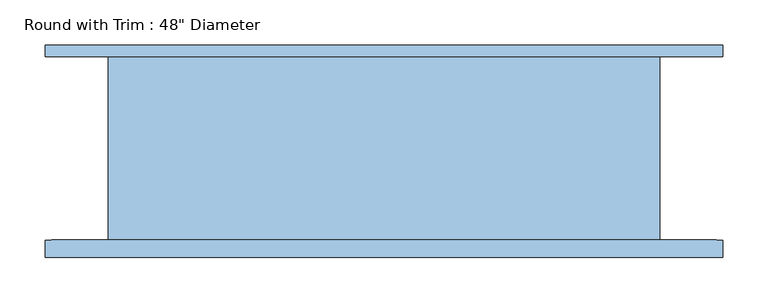
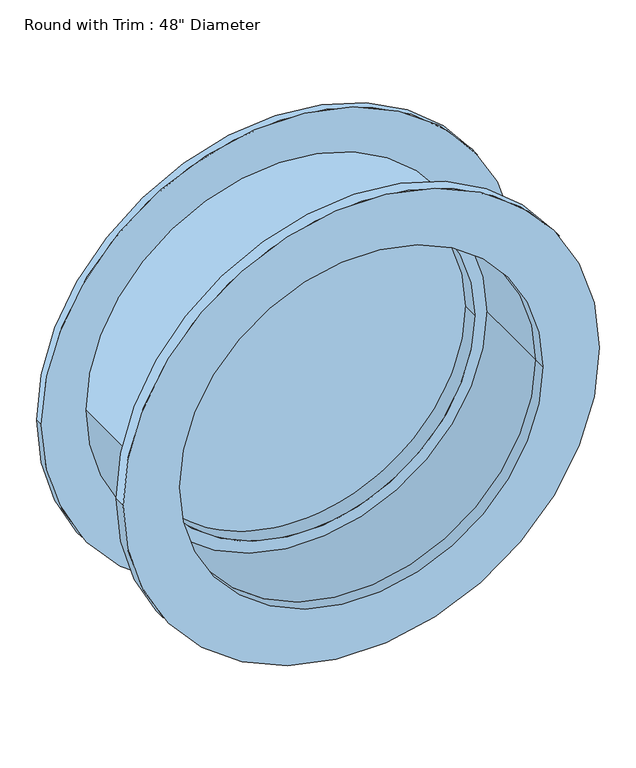
"""IFC4 building model written with IfcOpenShell, lengths in millimetres: window geometry."""

from ifc_helpers import new_model, si_unit, point, frame, frame_2d, origin, place, context, project, spatial, circle_curve, trimmed, segment, composite_curve, outline, extrude, source, transform, mapped, element, save


def window_3923817a(model_context):
    return source(origin(), model_context, "Body", "SweptSolid", [
        extrude(outline(composite_curve([segment(trimmed(circle_curve(frame_2d((914.4, -152.4)), 374.65), [point((914.4, -527.05))], [point((914.4, 222.25))], False, "CARTESIAN"), True, "CONTINUOUS"), segment(trimmed(circle_curve(frame_2d((914.4, -152.4)), 374.65), [point((914.4, 222.25))], [point((914.4, -527.05))], False, "CARTESIAN"), True, "CONTINUOUS")], self_intersect=False), holes=[composite_curve([segment(trimmed(circle_curve(frame_2d((914.4, -152.4)), 285.75), [point((914.4, -438.15))], [point((914.4, 133.35))], True, "CARTESIAN"), True, "CONTINUOUS"), segment(trimmed(circle_curve(frame_2d((914.4, -152.4)), 285.75), [point((914.4, 133.35))], [point((914.4, -438.15))], True, "CARTESIAN"), True, "CONTINUOUS")], self_intersect=False)]), frame((0.0, -120.65, 0.0), z_axis=(0.0, 1.0, 0.0), x_axis=(0.0, 0.0, 1.0)), (0.0, 0.0, 1.0), 19.05),
        extrude(outline(composite_curve([segment(trimmed(circle_curve(frame_2d((914.4, -152.4)), 374.65), [point((914.4, -527.05))], [point((914.4, 222.25))], False, "CARTESIAN"), True, "CONTINUOUS"), segment(trimmed(circle_curve(frame_2d((914.4, -152.4)), 374.65), [point((914.4, 222.25))], [point((914.4, -527.05))], False, "CARTESIAN"), True, "CONTINUOUS")], self_intersect=False), holes=[composite_curve([segment(trimmed(circle_curve(frame_2d((914.4, -152.4)), 285.75), [point((914.4, -438.15))], [point((914.4, 133.35))], True, "CARTESIAN"), True, "CONTINUOUS"), segment(trimmed(circle_curve(frame_2d((914.4, -152.4)), 285.75), [point((914.4, 133.35))], [point((914.4, -438.15))], True, "CARTESIAN"), True, "CONTINUOUS")], self_intersect=False)]), frame((0.0, 101.6, 0.0), z_axis=(0.0, 1.0, 0.0), x_axis=(0.0, 0.0, 1.0)), (0.0, 0.0, 1.0), 12.7),
        extrude(outline(composite_curve([segment(trimmed(circle_curve(frame_2d((914.4, -152.4)), 266.7), [point((914.4, -419.1))], [point((914.4, 114.3))], False, "CARTESIAN"), True, "CONTINUOUS"), segment(trimmed(circle_curve(frame_2d((914.4, -152.4)), 266.7), [point((914.4, 114.3))], [point((914.4, -419.1))], False, "CARTESIAN"), True, "CONTINUOUS")], self_intersect=False)), frame((0.0, 57.15, 0.0), z_axis=(0.0, 1.0, 0.0), x_axis=(0.0, 0.0, 1.0)), (0.0, 0.0, 1.0), 12.7),
        extrude(outline(composite_curve([segment(trimmed(circle_curve(frame_2d((914.4, -152.4)), 285.75), [point((914.4, -438.15))], [point((914.4, 133.35))], False, "CARTESIAN"), True, "CONTINUOUS"), segment(trimmed(circle_curve(frame_2d((914.4, -152.4)), 285.75), [point((914.4, 133.35))], [point((914.4, -438.15))], False, "CARTESIAN"), True, "CONTINUOUS")], self_intersect=False), holes=[composite_curve([segment(trimmed(circle_curve(frame_2d((914.4, -152.4)), 266.7), [point((914.4, -419.1))], [point((914.4, 114.3))], True, "CARTESIAN"), True, "CONTINUOUS"), segment(trimmed(circle_curve(frame_2d((914.4, -152.4)), 266.7), [point((914.4, 114.3))], [point((914.4, -419.1))], True, "CARTESIAN"), True, "CONTINUOUS")], self_intersect=False)]), frame((0.0, 31.75, 0.0), z_axis=(0.0, 1.0, 0.0), x_axis=(0.0, 0.0, 1.0)), (0.0, 0.0, 1.0), 50.8),
        extrude(outline(composite_curve([segment(trimmed(circle_curve(frame_2d((914.4, -152.4)), 304.8), [point((914.4, -457.2))], [point((914.4, 152.4))], False, "CARTESIAN"), True, "CONTINUOUS"), segment(trimmed(circle_curve(frame_2d((914.4, -152.4)), 304.8), [point((914.4, 152.4))], [point((914.4, -457.2))], False, "CARTESIAN"), True, "CONTINUOUS")], self_intersect=False), holes=[composite_curve([segment(trimmed(circle_curve(frame_2d((914.4, -152.4)), 285.75), [point((914.4, -438.15))], [point((914.4, 133.35))], True, "CARTESIAN"), True, "CONTINUOUS"), segment(trimmed(circle_curve(frame_2d((914.4, -152.4)), 285.75), [point((914.4, 133.35))], [point((914.4, -438.15))], True, "CARTESIAN"), True, "CONTINUOUS")], self_intersect=False)]), frame((0.0, -101.6, 0.0), z_axis=(0.0, 1.0, 0.0), x_axis=(0.0, 0.0, 1.0)), (0.0, 0.0, 1.0), 203.2),
    ])


if __name__ == "__main__":
    model = new_model("IFC4")
    model_context = context("Model", 3, world=origin())
    ifc_project = project(units=[si_unit("LENGTHUNIT", "METRE", prefix="MILLI")], contexts=[model_context])
    site = spatial("IfcSite", under=ifc_project)
    building = spatial("IfcBuilding", under=site)
    placement = place(None, origin())
    window_shape = window_3923817a(model_context)
    element("IfcWindow", 1, ObjectType="Round with Trim : 48\" Diameter", at=placement, inside=building, context=model_context, shape_type="MappedRepresentation", body=[
        mapped(window_shape, transform((0.0, 0.0, 0.0), x_axis=(1.0, 0.0, 0.0), y_axis=(0.0, 1.0, 0.0), z_axis=(0.0, 0.0, 1.0))),
    ])
    save(model, "model.ifc")

# Revit data of these elements
# Type "Round with Trim : 48\" Diameter"
#   Type Mark = "32"
#   Construction Type Id = "GSP4R"
#   Assembly Code = "B2020100"
#   Analytic Construction = "1/8 in Pilkington single glazing"
#   Visual Light Transmittance = 0.9
#   Solar Heat Gain Coefficient = 0.78
#   Heat Transfer Coefficient (U) = 0.6496 BTU/(h·ft²·°F)
#   Default Sill Height = 2' - 0"
#   Trim Projection - Ext. = 0' - 0 1/2"
#   Trim Projection - Int. = 0' - 0 3/4"
#   Trim Width - Exterior = 0' - 3 1/2"
#   Trim Width - Interior = 0' - 3 1/2"
#   Width = 2' - 0"
#   Define Thermal Properties by = 1
#   Glass Pane Material = Glass
#   Sash Material = Sash
#   Trim Exterior Material = Trim
#   Trim Interior Material = Trim
#   Wall Closure = (empty or 0)
# Element 1 (IfcWindow, "Round with Trim : 48\" Diameter")
#   Materials on its faces: "Trim", "Sash", "Glass"
# Materials
#   "Glass": class "Glass", colour RGB 0 128 192, transparency 0.75, Description = "Soda Lime Glass", Cost = 0
#   "Sash": class "Wood", colour RGB 224 178 126, transparency 0
#   "Trim": class "Wood", colour RGB 224 178 126, transparency 0
